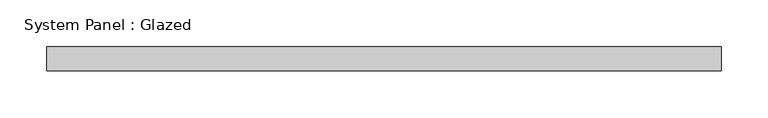
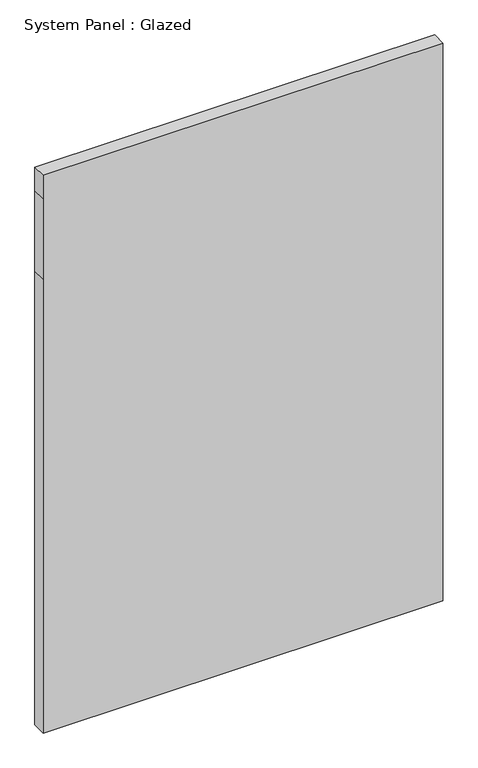
"""IFC4 building model written with IfcOpenShell, lengths in millimetres: plate geometry, System Panel : Glazed."""

from ifc_helpers import new_model, si_unit, frame, origin, place, context, project, spatial, polyline, outline, extrude, source, transform, mapped, element, save


def system_panel_glazed_917af8f4(model_context):
    return source(origin(), model_context, "Body", "SweptSolid", [
        extrude(outline(polyline([(0.0, -358.775), (0.0, 358.775), (861.2594531, 358.775), (1013.6594531, 358.775), (1058.1094531, 358.775), (1058.1094531, -358.775), (1013.6594531, -358.775), (861.2594531, -358.775), (0.0, -358.775)])), frame((0.0, 19.05, 0.0), z_axis=(0.0, 1.0, 0.0), x_axis=(0.0, 0.0, 1.0)), (0.0, 0.0, 1.0), 25.4),
    ])


if __name__ == "__main__":
    model = new_model("IFC4")
    model_context = context("Model", 3, world=origin())
    ifc_project = project(units=[si_unit("LENGTHUNIT", "METRE", prefix="MILLI")], contexts=[model_context])
    site = spatial("IfcSite", under=ifc_project)
    building = spatial("IfcBuilding", under=site)
    placement = place(None, origin())
    system_panel_glazed_shape = system_panel_glazed_917af8f4(model_context)
    element("IfcPlate", 1, ObjectType="System Panel : Glazed", at=placement, inside=building, context=model_context, shape_type="MappedRepresentation", body=[
        mapped(system_panel_glazed_shape, transform((0.0, 0.0, 0.0), x_axis=(1.0, 0.0, 0.0), y_axis=(0.0, 1.0, 0.0), z_axis=(0.0, 0.0, 1.0))),
    ])
    save(model, "model.ifc")

# Revit data of these elements
# Type "System Panel : Glazed"
#   Construction Type Id = "GSP4R"
#   Analytic Construction = "1/8 in Pilkington single glazing"
#   Visual Light Transmittance = 0.9
#   Solar Heat Gain Coefficient = 0.86
#   Heat Transfer Coefficient (U) = 1.18115 BTU/(h·ft²·°F)
#   Define Thermal Properties by = 1
# Element 1 (IfcPlate, "System Panel : Glazed")
#   Materials on its faces: "Glass"
# Materials
#   "Glass": class "Glass", colour RGB 0 128 192, transparency 0.75, Description = "Soda Lime Glass", Cost = 0
